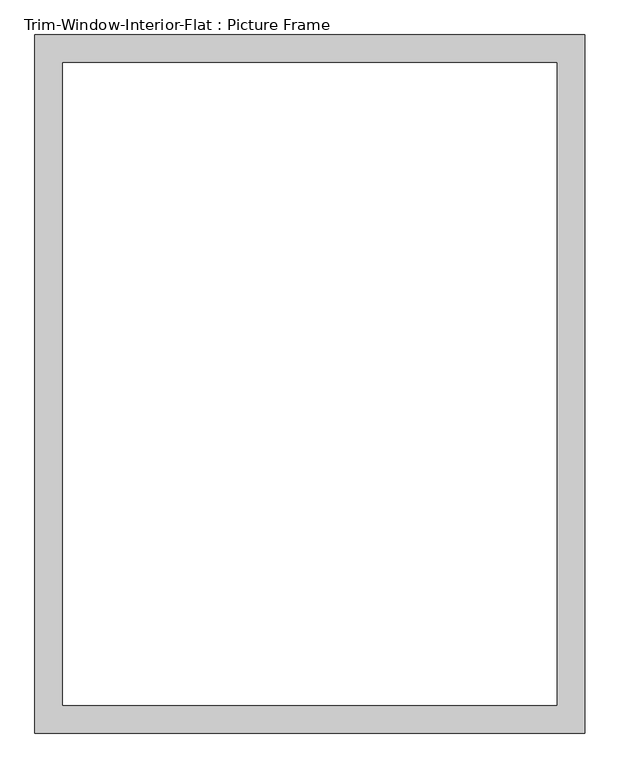
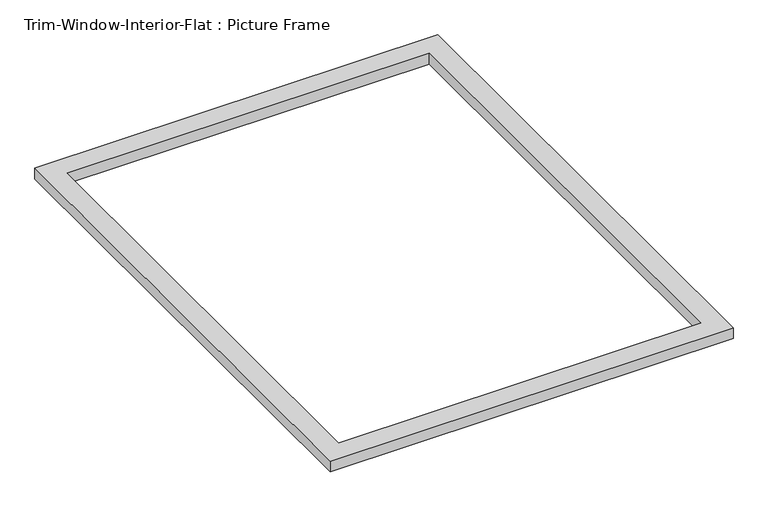
"""IFC4 building model written with IfcOpenShell, lengths in millimetres: proxy geometry, Trim-Window-Interior-Flat : Picture Frame."""

from ifc_helpers import new_model, si_unit, origin, origin_with_axes, place, context, project, spatial, polyline, outline, extrude, source, transform, mapped, element, save


def trim_window_interior_flat_picture_frame_dd064338(model_context):
    return source(origin(), model_context, "Body", "SweptSolid", [
        extrude(outline(polyline([(565.15, 44.45), (565.15, -1390.65), (-565.15, -1390.65), (-565.15, 44.45), (565.15, 44.45)]), holes=[polyline([(508.0, -12.7), (-508.0, -12.7), (-508.0, -1333.5), (508.0, -1333.5), (508.0, -12.7)])]), origin_with_axes(), (0.0, 0.0, 1.0), 31.75),
    ])


if __name__ == "__main__":
    model = new_model("IFC4")
    model_context = context("Model", 3, world=origin())
    ifc_project = project(units=[si_unit("LENGTHUNIT", "METRE", prefix="MILLI")], contexts=[model_context])
    site = spatial("IfcSite", under=ifc_project)
    building = spatial("IfcBuilding", under=site)
    placement = place(None, origin())
    trim_window_interior_flat_picture_frame_shape = trim_window_interior_flat_picture_frame_dd064338(model_context)
    element("IfcBuildingElementProxy", 1, Name="Trim-Window-Interior-Flat : Picture Frame", ObjectType="Trim-Window-Interior-Flat : Picture Frame", at=placement, inside=building, context=model_context, shape_type="MappedRepresentation", body=[
        mapped(trim_window_interior_flat_picture_frame_shape, transform((0.0, 0.0, 0.0), x_axis=(1.0, 0.0, 0.0), y_axis=(0.0, 1.0, 0.0), z_axis=(0.0, 0.0, 1.0))),
    ])
    save(model, "model.ifc")

# Revit data of these elements
# Type "Trim-Window-Interior-Flat : Picture Frame"
#   Trim Thickness_Picture Frame = 0' - 1 1/4"
#   Trim Width = 0' - 2 1/4"
#   Trim Thickness_with Sill = 0' - 0 3/4"
#   Sill Thickness = 0' - 1 1/4"
#   Opening Width [instance default] = 2' - 0"
#   Opening Height [instance default] = 3' - 0"
#   Default Elevation = 4' - 0"
#   Sill = no
#   Picture Frame = yes
#   Trim Material [instance default] = none
# Element 1 (IfcBuildingElementProxy, "Trim-Window-Interior-Flat : Picture Frame")
#   Opening Width = 3' - 5"
#   Opening Height = 4' - 5"
#   Trim Material = Wood - Stained
#   Materials on its faces: "Wood - Stained"
# Materials
#   "Wood - Stained": class "Wood", colour RGB 224 178 126, transparency 0, Cost = 0
